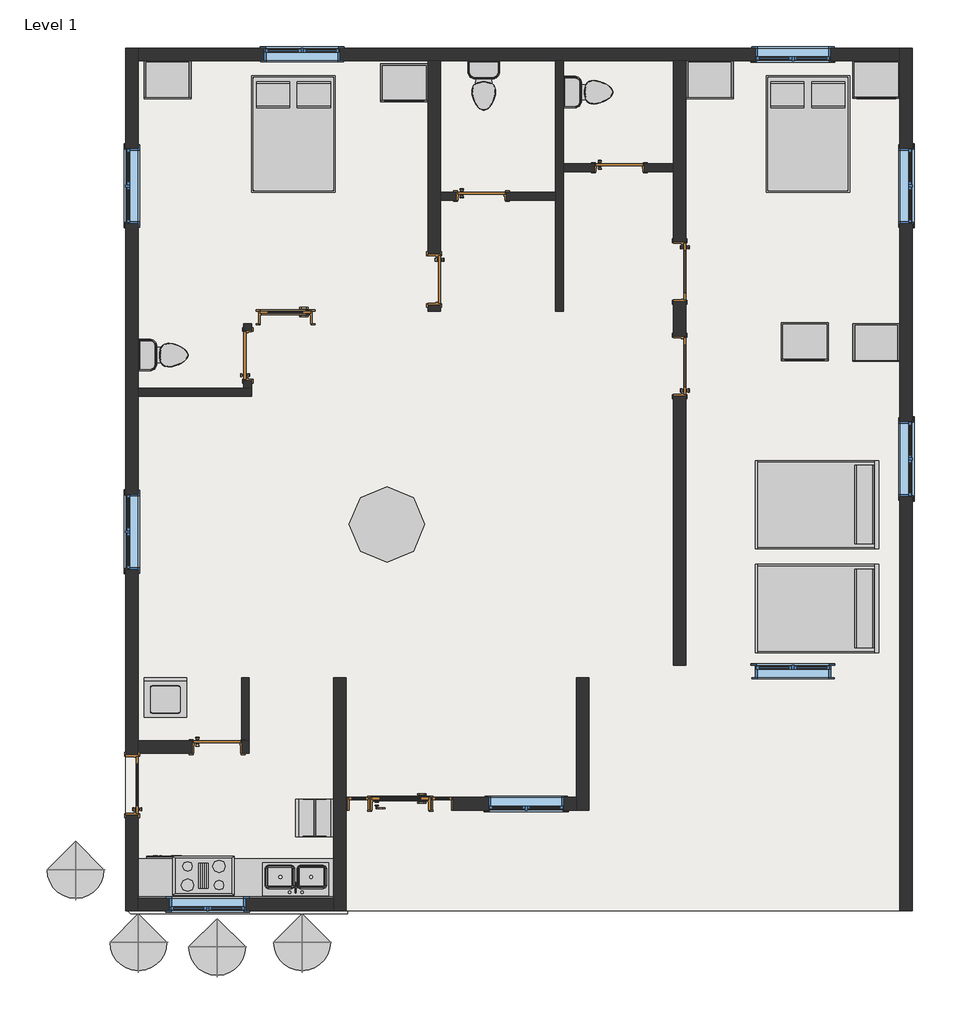
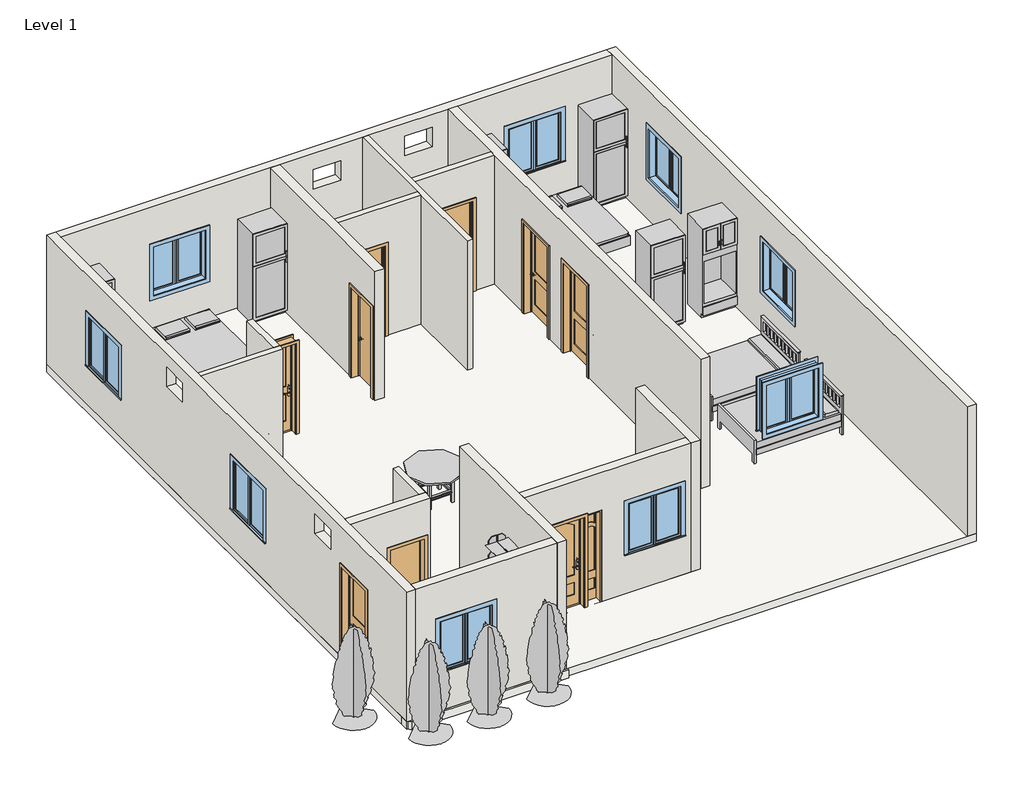
# One storey, incomplete: 16 walls, 13 doors, 12 furniture elements, 9 windows, 4 flow terminals, 4 geographic elements, 4 proxies, 3 slabs.
"""IFC4 building model written with IfcOpenShell, lengths in millimetres."""

from ifc_helpers import new_model, si_unit, frame, origin, place, context, project, spatial, polyline, outline, extrude, faceted_brep, transform, mapped, element, save
from components import proxy_a120491f, proxy_45b28599, proxy_279d5ef4, proxy_718fa39f, door_c3736dc5, door_823c627a, door_4a215221, door_6f959a6d, door_387d6dd4, door_interior_single_flush_panel_wood_df77f4d3, door_715cd483, entry_door_handle_standard_87575fd4, flow_terminal_a53be723, toilet_domestic_3d_toilet_domestic_3d_f7549cf7, toilet_domestic_3d_toilet_domestic_3d_183bbd19, furniture_c8abb964, furniture_096e7f55, furniture_23ec23c8, furniture_7060ebe6, furniture_fb6977ac, furniture_7f1a6afb, rpc_tree_conifer_chinese_juniper_7_1b9786cd, window_0862ab64, window_3a1167bf

model = new_model("IFC4")

# Units and contexts
model_context = context("Model", 3, world=origin())
ifc_project = project(units=[si_unit("LENGTHUNIT", "METRE", prefix="MILLI")], contexts=[model_context])

# Site, building, storey
site = spatial("IfcSite", under=ifc_project)
building = spatial("IfcBuilding", under=site)
storey = spatial("IfcBuildingStorey", under=building, Name="Level 1", Elevation=0.0)

# Proxies
placement = place(None, origin())
proxy_shape = proxy_a120491f(model_context)
element("IfcBuildingElementProxy", 1, Name="Cook Top-4 Unit : 42\" x 22\"", ObjectType="Cook Top-4 Unit : 42\" x 22\"", at=placement, inside=storey, context=model_context, shape_type="MappedRepresentation", body=[
    mapped(proxy_shape, transform((-17247.6111572, -428.8767698, 152.4), x_axis=(1.0, 0.0, 0.0), y_axis=(0.0, 1.0, 0.0), z_axis=(0.0, 0.0, 1.0))),
])
proxy_2_shape = proxy_45b28599(model_context)
element("IfcBuildingElementProxy", 2, Name="Dishwasher : 24\" x 24\" x 34\"", ObjectType="Dishwasher : 24\" x 24\" x 34\"", at=placement, inside=storey, context=model_context, shape_type="MappedRepresentation", body=[
    mapped(proxy_2_shape, transform((-17477.5286257, -168.2763346, 0.0), x_axis=(-1.0000000000000004, 0.0, 0.0), y_axis=(0.0, -1.0000000000000004, 0.0), z_axis=(0.0, 0.0, 1.0))),
])
proxy_3_shape = proxy_279d5ef4(model_context)
element("IfcBuildingElementProxy", 3, Name="Stack Shelving : 36\" x 90\"", ObjectType="Stack Shelving : 36\" x 90\"", at=placement, inside=storey, context=model_context, shape_type="MappedRepresentation", body=[
    mapped(proxy_3_shape, transform((-15450.5611572, 504.5732302, 0.0), x_axis=(0.0, 1.0000000000000002, 0.0), y_axis=(-1.0000000000000002, 0.0, 0.0), z_axis=(0.0, 0.0, 1.0))),
])
proxy_4_shape = proxy_718fa39f(model_context)
element("IfcBuildingElementProxy", 4, Name="Washer : 27\" x 25\" x 35\"", ObjectType="Washer : 27\" x 25\" x 35\"", at=placement, inside=storey, context=model_context, shape_type="MappedRepresentation", body=[
    mapped(proxy_4_shape, transform((-18280.2635627, 2168.5236654, 0.0), x_axis=(1.0, 0.0, 0.0), y_axis=(0.0, 1.0, 0.0), z_axis=(0.0, 0.0, 1.0))),
])

# Doors
door_shape = door_c3736dc5(model_context)
element("IfcDoor", 5, ObjectType="12\" x 84\"", at=placement, inside=storey, context=model_context, shape_type="MappedRepresentation", body=[
    mapped(door_shape, transform((-14739.3611572, 736.3482302, 0.0), x_axis=(1.0, 0.0, 0.0), y_axis=(0.0, 1.0, 0.0), z_axis=(0.0, 0.0, 1.0))),
])
element("IfcDoor", 6, ObjectType="12\" x 84\"", at=placement, inside=storey, context=model_context, shape_type="MappedRepresentation", body=[
    mapped(door_shape, transform((-13393.1611572, 736.3482302, 0.0), x_axis=(1.0, 0.0, 0.0), y_axis=(0.0, 1.0, 0.0), z_axis=(0.0, 0.0, 1.0))),
])
door_2_shape = door_823c627a(model_context)
element("IfcDoor", 7, ObjectType="32\" x 84\"", at=placement, inside=storey, context=model_context, shape_type="MappedRepresentation", body=[
    mapped(door_2_shape, transform((-15920.4611572, 8584.9482302, 0.0), x_axis=(1.0, 0.0, 0.0), y_axis=(0.0, 1.0, 0.0), z_axis=(0.0, 0.0, 1.0))),
])
door_3_shape = door_4a215221(model_context)
element("IfcDoor", 8, ObjectType="36\" x 84\"", at=placement, inside=storey, context=model_context, shape_type="MappedRepresentation", body=[
    mapped(door_3_shape, transform((-14066.2611572, 736.3482302, 0.0), x_axis=(1.0, 0.0, 0.0), y_axis=(0.0, 1.0, 0.0), z_axis=(0.0, 0.0, 1.0))),
])
door_4_shape = door_6f959a6d(model_context)
element("IfcDoor", 9, ObjectType="Door-Interior-Single-2_Panel-Wood : 36\" x 84\"", at=placement, inside=storey, context=model_context, shape_type="MappedRepresentation", body=[
    mapped(door_4_shape, transform((-9554.5861572, 9318.3732302, 0.0), x_axis=(0.0, -1.0, 0.0), y_axis=(1.0, 0.0, 0.0), z_axis=(0.0, 0.0, 1.0))),
])
door_5_shape = door_387d6dd4(model_context)
element("IfcDoor", 10, ObjectType="Door-Interior-Single-2_Panel-Wood : 36\" x 84\"", at=placement, inside=storey, context=model_context, shape_type="MappedRepresentation", body=[
    mapped(door_5_shape, transform((-9554.5861572, 7794.3732302, 0.0), x_axis=(0.0, 1.0, 0.0), y_axis=(-1.0, 0.0, 0.0), z_axis=(0.0, 0.0, 1.0))),
])
element("IfcDoor", 11, ObjectType="Door-Interior-Single-2_Panel-Wood : 36\" x 84\"", at=placement, inside=storey, context=model_context, shape_type="MappedRepresentation", body=[
    mapped(door_5_shape, transform((-18393.7861572, 1037.9732302, 0.0), x_axis=(0.0, 1.0, 0.0), y_axis=(-1.0, 0.0, 0.0), z_axis=(0.0, 0.0, 1.0))),
])
door_interior_single_flush_panel_wood_shape = door_interior_single_flush_panel_wood_df77f4d3(model_context)
element("IfcDoor", 12, ObjectType="Door-Interior-Single-Flush_Panel-Wood", at=placement, inside=storey, context=model_context, shape_type="MappedRepresentation", body=[
    mapped(door_interior_single_flush_panel_wood_shape, transform((-16533.2361572, 7965.8232302, 0.0), x_axis=(0.0, 1.0, 0.0), y_axis=(-1.0, 0.0, 0.0), z_axis=(0.0, 0.0, 1.0))),
])
element("IfcDoor", 13, ObjectType="Door-Interior-Single-Flush_Panel-Wood", at=placement, inside=storey, context=model_context, shape_type="MappedRepresentation", body=[
    mapped(door_interior_single_flush_panel_wood_shape, transform((-12758.1611572, 10540.7482302, 0.0), x_axis=(1.0, 0.0, 0.0), y_axis=(0.0, 1.0, 0.0), z_axis=(0.0, 0.0, 1.0))),
])
element("IfcDoor", 14, ObjectType="Door-Interior-Single-Flush_Panel-Wood", at=placement, inside=storey, context=model_context, shape_type="MappedRepresentation", body=[
    mapped(door_interior_single_flush_panel_wood_shape, transform((-10529.3111572, 10997.9482302, 0.0), x_axis=(1.0, 0.0, 0.0), y_axis=(0.0, 1.0, 0.0), z_axis=(0.0, 0.0, 1.0))),
])
door_6_shape = door_715cd483(model_context)
element("IfcDoor", 15, ObjectType="Door-Interior-Single-Flush_Panel-Wood", at=placement, inside=storey, context=model_context, shape_type="MappedRepresentation", body=[
    mapped(door_6_shape, transform((-13516.9861572, 9191.3732302, 0.0), x_axis=(0.0, -1.0, 0.0), y_axis=(1.0, 0.0, 0.0), z_axis=(0.0, 0.0, 1.0))),
])
element("IfcDoor", 16, ObjectType="Door-Interior-Single-Flush_Panel-Wood : 30\" x 84\"", at=placement, inside=storey, context=model_context, shape_type="MappedRepresentation", body=[
    mapped(door_6_shape, transform((-17025.3611572, 1650.7482302, 0.0), x_axis=(1.0, 0.0, 0.0), y_axis=(0.0, 1.0, 0.0), z_axis=(0.0, 0.0, 1.0))),
])
entry_door_handle_standard_shape = entry_door_handle_standard_87575fd4(model_context)
element("IfcDoor", 17, ObjectType="Entry Door Handle : Standard", at=placement, inside=storey, context=model_context, shape_type="MappedRepresentation", body=[
    mapped(entry_door_handle_standard_shape, transform((-14447.2611572, 733.1732302, 914.4), x_axis=(1.0, 0.0, 0.0), y_axis=(0.0, 1.0, 0.0), z_axis=(0.0, 0.0, 1.0))),
])

# Flow terminals
flow_terminal_shape = flow_terminal_a53be723(model_context)
element("IfcFlowTerminal", 18, ObjectType="Sink Kitchen-Double : 42\" x 21\"", at=placement, inside=storey, context=model_context, shape_type="MappedRepresentation", body=[
    mapped(flow_terminal_shape, transform((-15739.6719166, -483.6813687, 0.0), x_axis=(-1.0, 0.0, 0.0), y_axis=(0.0, -1.0, 0.0), z_axis=(0.0, 0.0, 1.0))),
])
toilet_domestic_3d_toilet_domestic_3d_shape = toilet_domestic_3d_toilet_domestic_3d_f7549cf7(model_context)
toilet_domestic_3d_toilet_domestic_3d_2_shape = toilet_domestic_3d_toilet_domestic_3d_183bbd19(model_context)
element("IfcFlowTerminal", 19, ObjectType="Toilet-Domestic-3D : Toilet-Domestic-3D", at=placement, inside=storey, context=model_context, shape_type="MappedRepresentation", body=[
    mapped(toilet_domestic_3d_toilet_domestic_3d_shape, transform((-17800.6651298, 7972.1732302, 0.0), x_axis=(0.0, 1.0000000000000002, 0.0), y_axis=(-1.0000000000000002, 0.0, 0.0), z_axis=(0.0, 0.0, 1.0))),
    mapped(toilet_domestic_3d_toilet_domestic_3d_2_shape, transform((-17800.6651298, 7972.1732302, 0.0), x_axis=(0.0, 1.0000000000000002, 0.0), y_axis=(-1.0000000000000002, 0.0, 0.0), z_axis=(0.0, 0.0, 1.0))),
])
element("IfcFlowTerminal", 20, ObjectType="Toilet-Domestic-3D : Toilet-Domestic-3D", at=placement, inside=storey, context=model_context, shape_type="MappedRepresentation", body=[
    mapped(toilet_domestic_3d_toilet_domestic_3d_shape, transform((-12720.0611572, 12227.2772028, 0.0), x_axis=(1.0000000000000007, 0.0, 0.0), y_axis=(0.0, 1.0000000000000007, 0.0), z_axis=(0.0, 0.0, 1.0))),
    mapped(toilet_domestic_3d_toilet_domestic_3d_2_shape, transform((-12720.0611572, 12227.2772028, 0.0), x_axis=(1.0000000000000007, 0.0, 0.0), y_axis=(0.0, 1.0000000000000007, 0.0), z_axis=(0.0, 0.0, 1.0))),
])
element("IfcFlowTerminal", 21, ObjectType="Toilet-Domestic-3D : Toilet-Domestic-3D", at=placement, inside=storey, context=model_context, shape_type="MappedRepresentation", body=[
    mapped(toilet_domestic_3d_toilet_domestic_3d_shape, transform((-10942.6651298, 12213.9732302, 0.0), x_axis=(0.0, 1.0000000000000002, 0.0), y_axis=(-1.0000000000000002, 0.0, 0.0), z_axis=(0.0, 0.0, 1.0))),
    mapped(toilet_domestic_3d_toilet_domestic_3d_2_shape, transform((-10942.6651298, 12213.9732302, 0.0), x_axis=(0.0, 1.0000000000000002, 0.0), y_axis=(-1.0000000000000002, 0.0, 0.0), z_axis=(0.0, 0.0, 1.0))),
])

# Furniture
furniture_shape = furniture_c8abb964(model_context)
element("IfcFurniture", 22, ObjectType="Bed-Box : Double 53\" x 74\"", at=placement, inside=storey, context=model_context, shape_type="MappedRepresentation", body=[
    mapped(furniture_shape, transform((-16132.6136162, 11775.3027384, 0.0), x_axis=(1.0, 0.0, 0.0), y_axis=(0.0, 1.0, 0.0), z_axis=(0.0, 0.0, 1.0))),
])
element("IfcFurniture", 23, ObjectType="Bed-Box : Double 53\" x 74\"", at=placement, inside=storey, context=model_context, shape_type="MappedRepresentation", body=[
    mapped(furniture_shape, transform((-7826.8136162, 11775.3027384, 0.0), x_axis=(1.0, 0.0, 0.0), y_axis=(0.0, 1.0, 0.0), z_axis=(0.0, 0.0, 1.0))),
])
furniture_2_shape = furniture_096e7f55(model_context)
element("IfcFurniture", 24, ObjectType="Bed-Shaker : Double 56\" x 78\"", at=placement, inside=storey, context=model_context, shape_type="MappedRepresentation", body=[
    mapped(furniture_2_shape, transform((-6357.3611572, 3863.7232302, 0.0), x_axis=(0.0, -1.0000000000000002, 0.0), y_axis=(1.0000000000000002, 0.0, 0.0), z_axis=(0.0, 0.0, 1.0))),
])
element("IfcFurniture", 25, ObjectType="Bed-Shaker : Double 56\" x 78\"", at=placement, inside=storey, context=model_context, shape_type="MappedRepresentation", body=[
    mapped(furniture_2_shape, transform((-6357.3611572, 5540.1232302, 0.0), x_axis=(0.0, -1.0000000000000002, 0.0), y_axis=(1.0000000000000002, 0.0, 0.0), z_axis=(0.0, 0.0, 1.0))),
])
furniture_3_shape = furniture_23ec23c8(model_context)
element("IfcFurniture", 26, ObjectType="Counter Top w Sink : 24\" Depth", at=placement, inside=storey, context=model_context, shape_type="MappedRepresentation", body=[
    mapped(furniture_3_shape, transform((-16346.2234522, -790.8267698, 0.0), x_axis=(-1.0, 0.0, 0.0), y_axis=(0.0, -1.0, 0.0), z_axis=(0.0, 0.0, 1.0))),
])
furniture_4_shape = furniture_7060ebe6(model_context)
element("IfcFurniture", 27, ObjectType="Table-Dining Round w Chairs : 36\" Diameter", at=placement, inside=storey, context=model_context, shape_type="MappedRepresentation", body=[
    mapped(furniture_4_shape, transform((-14385.8431244, 5426.5519187, 0.0), x_axis=(1.0, 0.0, 0.0), y_axis=(0.0, 1.0, 0.0), z_axis=(0.0, 0.0, 1.0))),
])
furniture_5_shape = furniture_fb6977ac(model_context)
element("IfcFurniture", 28, ObjectType="Tall Cabinet-2 Door-Built in : 30\"", at=placement, inside=storey, context=model_context, shape_type="MappedRepresentation", body=[
    mapped(furniture_5_shape, transform((-17844.1988621, 12721.9732302, 0.0), x_axis=(1.0, 0.0, 0.0), y_axis=(0.0, 1.0, 0.0), z_axis=(0.0, 0.0, 1.0))),
])
element("IfcFurniture", 29, ObjectType="Tall Cabinet-2 Door-Built in : 30\"", at=placement, inside=storey, context=model_context, shape_type="MappedRepresentation", body=[
    mapped(furniture_5_shape, transform((-9093.8988621, 12721.9732302, 0.0), x_axis=(1.0, 0.0, 0.0), y_axis=(0.0, 1.0, 0.0), z_axis=(0.0, 0.0, 1.0))),
])
element("IfcFurniture", 30, ObjectType="Tall Cabinet-2 Door-Built in : 30\"", at=placement, inside=storey, context=model_context, shape_type="MappedRepresentation", body=[
    mapped(furniture_5_shape, transform((-6401.4988621, 8480.1732302, 0.0), x_axis=(1.0, 0.0, 0.0), y_axis=(0.0, 1.0, 0.0), z_axis=(0.0, 0.0, 1.0))),
])
furniture_6_shape = furniture_7f1a6afb(model_context)
element("IfcFurniture", 31, ObjectType="Tall Cabinet-Single Door(2) : 30\"", at=placement, inside=storey, context=model_context, shape_type="MappedRepresentation", body=[
    mapped(furniture_6_shape, transform((-7557.1988621, 8492.8732302, 0.0), x_axis=(1.0000000000000002, 0.0, 0.0), y_axis=(0.0, 1.0000000000000002, 0.0), z_axis=(0.0, 0.0, 1.0))),
])
element("IfcFurniture", 32, ObjectType="Tall Cabinet-Single Door(2) : 30\"", at=placement, inside=storey, context=model_context, shape_type="MappedRepresentation", body=[
    mapped(furniture_6_shape, transform((-6401.4988621, 12721.9732302, 0.0), x_axis=(1.0, 0.0, 0.0), y_axis=(0.0, 1.0, 0.0), z_axis=(0.0, 0.0, 1.0))),
])
element("IfcFurniture", 33, ObjectType="Tall Cabinet-Single Door(2) : 30\"", at=placement, inside=storey, context=model_context, shape_type="MappedRepresentation", body=[
    mapped(furniture_6_shape, transform((-14021.4988621, 12671.1732302, 0.0), x_axis=(1.0, 0.0, 0.0), y_axis=(0.0, 1.0, 0.0), z_axis=(0.0, 0.0, 1.0))),
])

# Geographic elements
rpc_tree_conifer_chinese_juniper_7_shape = rpc_tree_conifer_chinese_juniper_7_1b9786cd(model_context)
element("IfcGeographicElement", 34, ObjectType="RPC Tree - Conifer : Chinese Juniper - 7'", at=placement, inside=storey, context=model_context, shape_type="MappedRepresentation", body=[
    mapped(rpc_tree_conifer_chinese_juniper_7_shape, transform((-18295.5578282, -1502.0267698, 0.0), x_axis=(1.0, 0.0, 0.0), y_axis=(0.0, 1.0, 0.0), z_axis=(0.0, 0.0, 1.0))),
])
element("IfcGeographicElement", 35, ObjectType="RPC Tree - Conifer : Chinese Juniper - 7'", at=placement, inside=storey, context=model_context, shape_type="MappedRepresentation", body=[
    mapped(rpc_tree_conifer_chinese_juniper_7_shape, transform((-17025.5578282, -1578.2267698, 0.0), x_axis=(1.0, 0.0, 0.0), y_axis=(0.0, 1.0, 0.0), z_axis=(0.0, 0.0, 1.0))),
])
element("IfcGeographicElement", 36, ObjectType="RPC Tree - Conifer : Chinese Juniper - 7'", at=placement, inside=storey, context=model_context, shape_type="MappedRepresentation", body=[
    mapped(rpc_tree_conifer_chinese_juniper_7_shape, transform((-15653.9578282, -1502.0267698, 0.0), x_axis=(1.0, 0.0, 0.0), y_axis=(0.0, 1.0, 0.0), z_axis=(0.0, 0.0, 1.0))),
])
element("IfcGeographicElement", 37, ObjectType="RPC Tree - Conifer : Chinese Juniper - 7'", at=placement, inside=storey, context=model_context, shape_type="MappedRepresentation", body=[
    mapped(rpc_tree_conifer_chinese_juniper_7_shape, transform((-19311.5578282, -333.6267698, 0.0), x_axis=(1.0, 0.0, 0.0), y_axis=(0.0, 1.0, 0.0), z_axis=(0.0, 0.0, 1.0))),
])

# Slabs
element("IfcSlab", 38, ObjectType="Generic - 12\"", at=placement, inside=storey, context=model_context, shape_type="SweptSolid", body=[
    extrude(outline(polyline([(-5798.5611572, 12925.1732302), (-5798.5611572, -790.8267698), (-5798.5611572, -994.0267698), (-18498.5611572, -994.0267698), (-18498.5611572, -790.8267698), (-18498.5611572, 12925.1732302), (-5798.5611572, 12925.1732302)])), frame((0.0, 0.0, -182.8601563), z_axis=(0.0, 0.0, 1.0), x_axis=(1.0, 0.0, 0.0)), (0.0, 0.0, 1.0), 182.8601563),
])
element("IfcSlab", 39, ObjectType="Generic - 12\"", at=placement, inside=storey, context=model_context, shape_type="SweptSolid", body=[
    extrude(outline(polyline([(-5798.5611572, 12925.1732302), (-5798.5611572, 2765.1732302), (-11018.2611572, 2765.1732302), (-11018.2611572, 631.5732302), (-14917.1611572, 631.5732302), (-14917.1611572, -1044.8267698), (-18422.3611572, -1044.8267698), (-18498.5611572, -968.6267698), (-18498.5611572, 12925.1732302), (-5798.5611572, 12925.1732302)])), frame((0.0, 0.0, -182.8601563), z_axis=(0.0, 0.0, 1.0), x_axis=(1.0, 0.0, 0.0)), (0.0, 0.0, 1.0), 182.8601563),
])
element("IfcSlab", 40, ObjectType="Generic - 12\"", at=placement, inside=storey, context=model_context, shape_type="SweptSolid", body=[
    extrude(outline(polyline([(-5798.5611572, 12925.1732302), (-5798.5611572, 2765.1732302), (-18498.5611572, 2765.1732302), (-18498.5611572, 12925.1732302), (-5798.5611572, 12925.1732302)])), frame((0.0, 0.0, -182.8601563), z_axis=(0.0, 0.0, 1.0), x_axis=(1.0, 0.0, 0.0)), (0.0, 0.0, 1.0), 182.8601563),
])

# Walls
element("IfcWall", 41, at=placement, inside=storey, context=model_context, shape_type="Brep", body=[
    faceted_brep([(-18295.3611572, 12721.9732302, 0.0), (-13621.7611572, 12721.9732302, 0.0), (-13418.5611572, 12721.9732302, 0.0), (-11564.3611572, 12721.9732302, 0.0), (-11437.3611572, 12721.9732302, 0.0), (-9659.3611572, 12721.9732302, 0.0), (-9456.1611572, 12721.9732302, 0.0), (-6001.7611572, 12721.9732302, 0.0), (-6001.7611572, 12721.9732302, 3048.0), (-9456.1611572, 12721.9732302, 3048.0), (-9659.3611572, 12721.9732302, 3048.0), (-11437.3611572, 12721.9732302, 3048.0), (-11564.3611572, 12721.9732302, 3048.0), (-13418.5611572, 12721.9732302, 3048.0), (-13621.7611572, 12721.9732302, 3048.0), (-18295.3611572, 12721.9732302, 3048.0), (-16263.3611572, 12721.9732302, 2133.6), (-15044.1611572, 12721.9732302, 2133.6), (-15044.1611572, 12721.9732302, 914.4), (-16263.3611572, 12721.9732302, 914.4), (-8338.5611572, 12721.9732302, 2133.6), (-7119.3611572, 12721.9732302, 2133.6), (-7119.3611572, 12721.9732302, 914.4), (-8338.5611572, 12721.9732302, 914.4), (-12053.3111572, 12721.9732302, 2667.0), (-12053.3111572, 12721.9732302, 2209.8), (-12662.9111572, 12721.9732302, 2209.8), (-12662.9111572, 12721.9732302, 2667.0), (-10624.5611572, 12721.9732302, 2743.2), (-10014.9611572, 12721.9732302, 2743.2), (-10014.9611572, 12721.9732302, 2286.0), (-10624.5611572, 12721.9732302, 2286.0), (-18295.3611572, 12925.1732302, 0.0), (-18295.3611572, 12925.1732302, 3048.0), (-6001.7611572, 12925.1732302, 3048.0), (-6001.7611572, 12925.1732302, 0.0), (-16263.3611572, 12925.1732302, 2133.6), (-16263.3611572, 12925.1732302, 914.4), (-15044.1611572, 12925.1732302, 914.4), (-15044.1611572, 12925.1732302, 2133.6), (-8338.5611572, 12925.1732302, 2133.6), (-8338.5611572, 12925.1732302, 914.4), (-7119.3611572, 12925.1732302, 914.4), (-7119.3611572, 12925.1732302, 2133.6), (-12053.3111572, 12925.1732302, 2667.0), (-12662.9111572, 12925.1732302, 2667.0), (-12662.9111572, 12925.1732302, 2209.8), (-12053.3111572, 12925.1732302, 2209.8), (-10624.5611572, 12925.1732302, 2743.2), (-10624.5611572, 12925.1732302, 2286.0), (-10014.9611572, 12925.1732302, 2286.0), (-10014.9611572, 12925.1732302, 2743.2)], [[[0, 1, 2, 3, 4, 5, 6, 7, 8, 9, 10, 11, 12, 13, 14, 15], [16, 17, 18, 19], [20, 21, 22, 23], [24, 25, 26, 27], [28, 29, 30, 31]], [[32, 33, 34, 35], [36, 37, 38, 39], [40, 41, 42, 43], [44, 45, 46, 47], [48, 49, 50, 51]], [[7, 6, 5, 4, 3, 2, 1, 0, 32, 35]], [[15, 14, 13, 12, 11, 10, 9, 8, 34, 33]], [[0, 15, 33, 32]], [[8, 7, 35, 34]], [[37, 36, 16, 19]], [[38, 37, 19, 18]], [[39, 38, 18, 17]], [[36, 39, 17, 16]], [[41, 40, 20, 23]], [[42, 41, 23, 22]], [[43, 42, 22, 21]], [[40, 43, 21, 20]], [[25, 24, 44, 47]], [[26, 25, 47, 46]], [[27, 26, 46, 45]], [[24, 27, 45, 44]], [[49, 48, 28, 31]], [[50, 49, 31, 30]], [[51, 50, 30, 29]], [[48, 51, 29, 28]]]),
])
element("IfcWall", 42, at=placement, inside=storey, context=model_context, shape_type="Brep", body=[
    faceted_brep([(-6001.7611572, 12925.1732302, 0.0), (-6001.7611572, 12721.9732302, 0.0), (-6001.7611572, 8683.3732302, 0.0), (-6001.7611572, 8480.1732302, 0.0), (-6001.7611572, 2968.3732302, 0.0), (-6001.7611572, 2765.1732302, 0.0), (-6001.7611572, -994.0267698, 0.0), (-6001.7611572, -994.0267698, 3048.0), (-6001.7611572, 2765.1732302, 3048.0), (-6001.7611572, 2968.3732302, 3048.0), (-6001.7611572, 8480.1732302, 3048.0), (-6001.7611572, 8683.3732302, 3048.0), (-6001.7611572, 12721.9732302, 3048.0), (-6001.7611572, 12925.1732302, 3048.0), (-6001.7611572, 10093.0732302, 2209.8), (-6001.7611572, 10093.0732302, 990.6), (-6001.7611572, 11312.2732302, 990.6), (-6001.7611572, 11312.2732302, 2209.8), (-6001.7611572, 5686.1732302, 2209.8), (-6001.7611572, 5686.1732302, 990.6), (-6001.7611572, 6905.3732302, 990.6), (-6001.7611572, 6905.3732302, 2209.8), (-5798.5611572, 12925.1732302, 0.0), (-5798.5611572, 12925.1732302, 3048.0), (-5798.5611572, -994.0267698, 3048.0), (-5798.5611572, -994.0267698, 0.0), (-5798.5611572, 10093.0732302, 2209.8), (-5798.5611572, 11312.2732302, 2209.8), (-5798.5611572, 11312.2732302, 990.6), (-5798.5611572, 10093.0732302, 990.6), (-5798.5611572, 5686.1732302, 2209.8), (-5798.5611572, 6905.3732302, 2209.8), (-5798.5611572, 6905.3732302, 990.6), (-5798.5611572, 5686.1732302, 990.6)], [[[0, 1, 2, 3, 4, 5, 6, 7, 8, 9, 10, 11, 12, 13], [14, 15, 16, 17], [18, 19, 20, 21]], [[22, 23, 24, 25], [26, 27, 28, 29], [30, 31, 32, 33]], [[6, 5, 4, 3, 2, 1, 0, 22, 25]], [[7, 6, 25, 24]], [[13, 12, 11, 10, 9, 8, 7, 24, 23]], [[0, 13, 23, 22]], [[15, 14, 26, 29]], [[16, 15, 29, 28]], [[17, 16, 28, 27]], [[14, 17, 27, 26]], [[19, 18, 30, 33]], [[20, 19, 33, 32]], [[21, 20, 32, 31]], [[18, 21, 31, 30]]]),
])
element("IfcWall", 43, ObjectType="Generic - 5\"", at=placement, inside=storey, context=model_context, shape_type="Brep", body=[
    faceted_brep([(-11564.3611572, 12721.9732302, 0.0), (-11564.3611572, 10601.0732302, 0.0), (-11564.3611572, 10474.0732302, 0.0), (-11564.3611572, 8683.3732302, 0.0), (-11564.3611572, 8683.3732302, 3048.0), (-11564.3611572, 10474.0732302, 3048.0), (-11564.3611572, 10601.0732302, 3048.0), (-11564.3611572, 12721.9732302, 3048.0), (-11437.3611572, 12721.9732302, 0.0), (-11437.3611572, 12721.9732302, 3048.0), (-11437.3611572, 11058.2732302, 3048.0), (-11437.3611572, 10931.2732302, 3048.0), (-11437.3611572, 8683.3732302, 3048.0), (-11437.3611572, 8683.3732302, 1325.7615426), (-11437.3611572, 8683.3732302, 0.0), (-11437.3611572, 10931.2732302, 0.0), (-11437.3611572, 11058.2732302, 0.0)], [[[0, 1, 2, 3, 4, 5, 6, 7]], [[8, 9, 10, 11, 12, 13, 14, 15, 16]], [[3, 2, 1, 0, 8, 16, 15, 14]], [[7, 6, 5, 4, 12, 11, 10, 9]], [[0, 7, 9, 8]], [[3, 14, 13, 12, 4]]]),
])
element("IfcWall", 44, ObjectType="Generic - 5\"", at=placement, inside=storey, context=model_context, shape_type="Brep", body=[
    faceted_brep([(-18295.3611572, 7311.7732302, 0.0), (-16466.5611572, 7311.7732302, 0.0), (-16466.5611572, 7311.7732302, 3048.0), (-18295.3611572, 7311.7732302, 3048.0), (-18295.3611572, 7438.7732302, 0.0), (-18295.3611572, 7438.7732302, 3048.0), (-16593.5611572, 7438.7732302, 3048.0), (-16466.5611572, 7438.7732302, 3048.0), (-16466.5611572, 7438.7732302, 0.0), (-16593.5611572, 7438.7732302, 0.0)], [[[0, 1, 2, 3]], [[4, 5, 6, 7, 8, 9]], [[1, 0, 4, 9, 8]], [[3, 2, 7, 6, 5]], [[0, 3, 5, 4]], [[2, 1, 8, 7]]]),
])
element("IfcWall", 45, ObjectType="Generic - 5\"", at=placement, inside=storey, context=model_context, shape_type="SweptSolid", body=[
    extrude(outline(polyline([(7438.7732302, 3048.0), (8480.1732302, 3048.0), (8480.1732302, 0.0), (8372.2232302, 0.0), (8372.2232302, 2159.0), (7559.4232302, 2159.0), (7559.4232302, 0.0), (7438.7732302, 0.0), (7438.7732302, 3048.0)])), frame((-16593.5611572, 0.0, 0.0), z_axis=(1.0, 0.0, 0.0), x_axis=(0.0, 1.0, 0.0)), (0.0, 0.0, 1.0), 127.0),
])
element("IfcWall", 46, ObjectType="Generic - 5\"", at=placement, inside=storey, context=model_context, shape_type="Brep", body=[
    faceted_brep([(-16631.6611572, 2765.1732302, 0.0), (-16631.6611572, 1749.1732302, 0.0), (-16631.6611572, 1749.1732302, 3048.0), (-16631.6611572, 2765.1732302, 3048.0), (-16504.6611572, 2765.1732302, 0.0), (-16504.6611572, 2765.1732302, 3048.0), (-16504.6611572, 1749.1732302, 3048.0), (-16504.6611572, 1749.1732302, 0.0), (-16618.9611572, 1749.1732302, 0.0)], [[[0, 1, 2, 3]], [[4, 5, 6, 7]], [[1, 0, 4, 7, 8]], [[3, 2, 6, 5]], [[2, 1, 8, 7, 6]], [[0, 3, 5, 4]]]),
])
element("IfcWall", 47, ObjectType="Generic - 5\"", at=placement, inside=storey, context=model_context, shape_type="SweptSolid", body=[
    extrude(outline(polyline([(3048.0, -9659.3611572), (3048.0, -11437.3611572), (0.0, -11437.3611572), (0.0, -10935.7111572), (2159.0, -10935.7111572), (2159.0, -10122.9111572), (0.0, -10122.9111572), (0.0, -9659.3611572), (3048.0, -9659.3611572)])), frame((0.0, 10931.2732302, 0.0), z_axis=(0.0, 1.0, 0.0), x_axis=(0.0, 0.0, 1.0)), (0.0, 0.0, 1.0), 127.0),
])
element("IfcWall", 48, ObjectType="Generic - 5\"", at=placement, inside=storey, context=model_context, shape_type="SweptSolid", body=[
    extrude(outline(polyline([(3048.0, -11564.3611572), (3048.0, -13418.5611572), (0.0, -13418.5611572), (0.0, -13164.5611572), (2159.0, -13164.5611572), (2159.0, -12351.7611572), (0.0, -12351.7611572), (0.0, -11564.3611572), (3048.0, -11564.3611572)])), frame((0.0, 10474.0732302, 0.0), z_axis=(0.0, 1.0, 0.0), x_axis=(0.0, 0.0, 1.0)), (0.0, 0.0, 1.0), 127.0),
])
element("IfcWall", 49, ObjectType="Generic - 8\"", at=placement, inside=storey, context=model_context, shape_type="Brep", body=[
    faceted_brep([(-13621.7611572, 8683.3732302, 3048.0), (-13621.7611572, 12721.9732302, 3048.0), (-13621.7611572, 12721.9732302, 0.0), (-13621.7611572, 9597.7732302, 0.0), (-13621.7611572, 9597.7732302, 2159.0), (-13621.7611572, 8784.9732302, 2159.0), (-13621.7611572, 8784.9732302, 0.0), (-13621.7611572, 8683.3732302, 0.0), (-13418.5611572, 12721.9732302, 3048.0), (-13418.5611572, 10601.0732302, 3048.0), (-13418.5611572, 10474.0732302, 3048.0), (-13418.5611572, 8683.3732302, 3048.0), (-13418.5611572, 8683.3732302, 0.0), (-13418.5611572, 8784.9732302, 0.0), (-13418.5611572, 8784.9732302, 2159.0), (-13418.5611572, 9597.7732302, 2159.0), (-13418.5611572, 9597.7732302, 0.0), (-13418.5611572, 10474.0732302, 0.0), (-13418.5611572, 10601.0732302, 0.0), (-13418.5611572, 12721.9732302, 0.0)], [[[0, 1, 2, 3, 4, 5, 6, 7]], [[8, 9, 10, 11, 12, 13, 14, 15, 16, 17, 18, 19]], [[2, 19, 18, 17, 16, 3]], [[12, 7, 6, 13]], [[1, 0, 11, 10, 9, 8]], [[2, 1, 8, 19]], [[0, 7, 12, 11]], [[5, 14, 13, 6]], [[14, 5, 4, 15]], [[15, 4, 3, 16]]]),
])
element("IfcWall", 50, ObjectType="Generic - 8\"", at=placement, inside=storey, context=model_context, shape_type="Brep", body=[
    faceted_brep([(-9659.3611572, 2968.3732302, 3048.0), (-9659.3611572, 8280.1770962, 3048.0), (-9659.3611572, 8454.7732302, 3048.0), (-9659.3611572, 8480.1732302, 3048.0), (-9659.3611572, 10931.2732302, 3048.0), (-9659.3611572, 11058.2732302, 3048.0), (-9659.3611572, 12721.9732302, 3048.0), (-9659.3611572, 12721.9732302, 0.0), (-9659.3611572, 11058.2732302, 0.0), (-9659.3611572, 10931.2732302, 0.0), (-9659.3611572, 9800.9732302, 0.0), (-9659.3611572, 9800.9732302, 2159.0), (-9659.3611572, 8835.7732302, 2159.0), (-9659.3611572, 8835.7732302, 0.0), (-9659.3611572, 8556.3732302, 0.0), (-9659.3611572, 8454.7732302, 0.0), (-9659.3611572, 8353.1732302, 0.0), (-9659.3611572, 8276.9732302, 0.0), (-9659.3611572, 8276.9732302, 2159.0), (-9659.3611572, 7311.7732302, 2159.0), (-9659.3611572, 7311.7732302, 0.0), (-9659.3611572, 2968.3732302, 0.0), (-9456.1611572, 12721.9732302, 3048.0), (-9456.1611572, 2968.3732302, 3048.0), (-9456.1611572, 2968.3732302, 0.0), (-9456.1611572, 7311.7732302, 0.0), (-9456.1611572, 7311.7732302, 2159.0), (-9456.1611572, 8276.9732302, 2159.0), (-9456.1611572, 8276.9732302, 0.0), (-9456.1611572, 8835.7732302, 0.0), (-9456.1611572, 8835.7732302, 2159.0), (-9456.1611572, 9800.9732302, 2159.0), (-9456.1611572, 9800.9732302, 0.0), (-9456.1611572, 12721.9732302, 0.0)], [[[0, 1, 2, 3, 4, 5, 6, 7, 8, 9, 10, 11, 12, 13, 14, 15, 16, 17, 18, 19, 20, 21]], [[22, 23, 24, 25, 26, 27, 28, 29, 30, 31, 32, 33]], [[7, 6, 22, 33]], [[0, 21, 24, 23]], [[12, 30, 29, 13]], [[30, 12, 11, 31]], [[31, 11, 10, 32]], [[27, 18, 17, 28]], [[18, 27, 26, 19]], [[19, 26, 25, 20]], [[10, 9, 8, 7, 33, 32]], [[13, 29, 28, 17, 16, 15, 14]], [[24, 21, 20, 25]], [[6, 5, 4, 3, 2, 1, 0, 23, 22]]]),
])
element("IfcWall", 51, ObjectType="Generic - 8\"", at=placement, inside=storey, context=model_context, shape_type="Brep", body=[
    faceted_brep([(-15145.7611572, 2765.1732302, 0.0), (-15145.7611572, -790.8267698, 0.0), (-15145.7611572, -994.0267698, 0.0), (-15145.7611572, -994.0267698, 3048.0), (-15145.7611572, -790.8267698, 3048.0), (-15145.7611572, 2765.1732302, 3048.0), (-14942.5611572, 2765.1732302, 0.0), (-14942.5611572, 2765.1732302, 3048.0), (-14942.5611572, 834.7732302, 3048.0), (-14942.5611572, 631.5732302, 3048.0), (-14942.5611572, -994.0267698, 3048.0), (-14942.5611572, -994.0267698, 0.0), (-14942.5611572, 631.5732302, 0.0), (-14942.5611572, 834.7732302, 0.0)], [[[0, 1, 2, 3, 4, 5]], [[6, 7, 8, 9, 10, 11, 12, 13]], [[2, 1, 0, 6, 13, 12, 11]], [[5, 4, 3, 10, 9, 8, 7]], [[3, 2, 11, 10]], [[0, 5, 7, 6]]]),
])
element("IfcWall", 52, ObjectType="Generic - 8\"", at=placement, inside=storey, context=model_context, shape_type="Brep", body=[
    faceted_brep([(-16504.6611572, 1545.9732302, 3048.0), (-18295.3611572, 1545.9732302, 3048.0), (-18295.3611572, 1545.9732302, 0.0), (-17431.7611572, 1545.9732302, 0.0), (-17431.7611572, 1545.9732302, 2159.0), (-16618.9611572, 1545.9732302, 2159.0), (-16618.9611572, 1545.9732302, 0.0), (-16504.6611572, 1545.9732302, 0.0), (-18295.3611572, 1749.1732302, 3048.0), (-16631.6611572, 1749.1732302, 3048.0), (-16504.6611572, 1749.1732302, 3048.0), (-16504.6611572, 1749.1732302, 0.0), (-16618.9611572, 1749.1732302, 0.0), (-16618.9611572, 1749.1732302, 2159.0), (-17431.7611572, 1749.1732302, 2159.0), (-17431.7611572, 1749.1732302, 0.0), (-18295.3611572, 1749.1732302, 0.0)], [[[0, 1, 2, 3, 4, 5, 6, 7]], [[8, 9, 10, 11, 12, 13, 14, 15, 16]], [[2, 16, 15, 3]], [[11, 7, 6, 12]], [[1, 0, 10, 9, 8]], [[2, 1, 8, 16]], [[0, 7, 11, 10]], [[5, 13, 12, 6]], [[13, 5, 4, 14]], [[14, 4, 3, 15]]]),
])
element("IfcWall", 53, ObjectType="a", at=placement, inside=storey, context=model_context, shape_type="Brep", body=[
    faceted_brep([(-18498.5611572, -994.0267698, 3048.0), (-18498.5611572, 12925.1732302, 3048.0), (-18498.5611572, 12925.1732302, 0.0), (-18498.5611572, 1520.5732302, 0.0), (-18498.5611572, 1520.5732302, 2159.0), (-18498.5611572, 555.3732302, 2159.0), (-18498.5611572, 555.3732302, 0.0), (-18498.5611572, -994.0267698, 0.0), (-18498.5611572, 5730.6232302, 2133.6), (-18498.5611572, 4511.4232302, 2133.6), (-18498.5611572, 4511.4232302, 914.4), (-18498.5611572, 5730.6232302, 914.4), (-18498.5611572, 11312.2732302, 2133.6), (-18498.5611572, 10093.0732302, 2133.6), (-18498.5611572, 10093.0732302, 914.4), (-18498.5611572, 11312.2732302, 914.4), (-18498.5611572, 8283.3232302, 2743.2), (-18498.5611572, 7673.7232302, 2743.2), (-18498.5611572, 7673.7232302, 2286.0), (-18498.5611572, 8283.3232302, 2286.0), (-18498.5611572, 2561.9732302, 2743.2), (-18498.5611572, 1952.3732302, 2743.2), (-18498.5611572, 1952.3732302, 2286.0), (-18498.5611572, 2561.9732302, 2286.0), (-18295.3611572, 12925.1732302, 3048.0), (-18295.3611572, 12721.9732302, 3048.0), (-18295.3611572, 8683.3732302, 3048.0), (-18295.3611572, 8480.1732302, 3048.0), (-18295.3611572, 7438.7732302, 3048.0), (-18295.3611572, 7311.7732302, 3048.0), (-18295.3611572, 2968.3732302, 3048.0), (-18295.3611572, 2765.1732302, 3048.0), (-18295.3611572, 1749.1732302, 3048.0), (-18295.3611572, 1545.9732302, 3048.0), (-18295.3611572, -790.8267698, 3048.0), (-18295.3611572, -994.0267698, 3048.0), (-18295.3611572, -994.0267698, 0.0), (-18295.3611572, -790.8267698, 0.0), (-18295.3611572, 555.3732302, 0.0), (-18295.3611572, 555.3732302, 2159.0), (-18295.3611572, 1520.5732302, 2159.0), (-18295.3611572, 1520.5732302, 0.0), (-18295.3611572, 1545.9732302, 0.0), (-18295.3611572, 1749.1732302, 0.0), (-18295.3611572, 2765.1732302, 0.0), (-18295.3611572, 2968.3732302, 0.0), (-18295.3611572, 7311.7732302, 0.0), (-18295.3611572, 7438.7732302, 0.0), (-18295.3611572, 8480.1732302, 0.0), (-18295.3611572, 8683.3732302, 0.0), (-18295.3611572, 12721.9732302, 0.0), (-18295.3611572, 12925.1732302, 0.0), (-18295.3611572, 5730.6232302, 2133.6), (-18295.3611572, 5730.6232302, 914.4), (-18295.3611572, 4511.4232302, 914.4), (-18295.3611572, 4511.4232302, 2133.6), (-18295.3611572, 11312.2732302, 2133.6), (-18295.3611572, 11312.2732302, 914.4), (-18295.3611572, 10093.0732302, 914.4), (-18295.3611572, 10093.0732302, 2133.6), (-18295.3611572, 8283.3232302, 2743.2), (-18295.3611572, 8283.3232302, 2286.0), (-18295.3611572, 7673.7232302, 2286.0), (-18295.3611572, 7673.7232302, 2743.2), (-18295.3611572, 2561.9732302, 2743.2), (-18295.3611572, 2561.9732302, 2286.0), (-18295.3611572, 1952.3732302, 2286.0), (-18295.3611572, 1952.3732302, 2743.2)], [[[0, 1, 2, 3, 4, 5, 6, 7], [8, 9, 10, 11], [12, 13, 14, 15], [16, 17, 18, 19], [20, 21, 22, 23]], [[24, 25, 26, 27, 28, 29, 30, 31, 32, 33, 34, 35, 36, 37, 38, 39, 40, 41, 42, 43, 44, 45, 46, 47, 48, 49, 50, 51], [52, 53, 54, 55], [56, 57, 58, 59], [60, 61, 62, 63], [64, 65, 66, 67]], [[2, 51, 50, 49, 48, 47, 46, 45, 44, 43, 42, 41, 3]], [[36, 7, 6, 38, 37]], [[1, 0, 35, 34, 33, 32, 31, 30, 29, 28, 27, 26, 25, 24]], [[2, 1, 24, 51]], [[0, 7, 36, 35]], [[40, 4, 3, 41]], [[4, 40, 39, 5]], [[5, 39, 38, 6]], [[53, 52, 8, 11]], [[54, 53, 11, 10]], [[55, 54, 10, 9]], [[52, 55, 9, 8]], [[57, 56, 12, 15]], [[58, 57, 15, 14]], [[59, 58, 14, 13]], [[56, 59, 13, 12]], [[61, 60, 16, 19]], [[62, 61, 19, 18]], [[63, 62, 18, 17]], [[60, 63, 17, 16]], [[65, 64, 20, 23]], [[66, 65, 23, 22]], [[67, 66, 22, 21]], [[64, 67, 21, 20]]]),
])
element("IfcWall", 54, ObjectType="aw", at=placement, inside=storey, context=model_context, shape_type="SweptSolid", body=[
    extrude(outline(polyline([(0.0, -18295.3611572), (0.0, -15145.7611572), (3048.0, -15145.7611572), (3048.0, -18295.3611572), (0.0, -18295.3611572)]), holes=[polyline([(2133.6, -17787.3611572), (2133.6, -16568.1611572), (914.4, -16568.1611572), (914.4, -17787.3611572), (2133.6, -17787.3611572)])]), frame((0.0, -994.0267698, 0.0), z_axis=(0.0, 1.0, 0.0), x_axis=(0.0, 0.0, 1.0)), (0.0, 0.0, 1.0), 203.2),
])
element("IfcWall", 55, ObjectType="dq", at=placement, inside=storey, context=model_context, shape_type="Brep", body=[
    faceted_brep([(-11221.4611572, 2765.1732302, 0.0), (-11221.4611572, 834.7732302, 0.0), (-11221.4611572, 631.5732302, 0.0), (-11221.4611572, 631.5732302, 3048.0), (-11221.4611572, 834.7732302, 3048.0), (-11221.4611572, 2765.1732302, 3048.0), (-11018.2611572, 2765.1732302, 0.0), (-11018.2611572, 2765.1732302, 3048.0), (-11018.2611572, 631.5732302, 3048.0), (-11018.2611572, 631.5732302, 0.0)], [[[0, 1, 2, 3, 4, 5]], [[6, 7, 8, 9]], [[2, 1, 0, 6, 9]], [[5, 4, 3, 8, 7]], [[0, 5, 7, 6]], [[3, 2, 9, 8]]]),
])
element("IfcWall", 56, ObjectType="dq", at=placement, inside=storey, context=model_context, shape_type="SweptSolid", body=[
    extrude(outline(polyline([(3048.0, -11221.4611572), (3048.0, -14942.5611572), (0.0, -14942.5611572), (0.0, -14917.1611572), (2159.0, -14917.1611572), (2159.0, -14561.5611572), (0.0, -14561.5611572), (0.0, -14548.8611572), (2159.0, -14548.8611572), (2159.0, -13583.6611572), (0.0, -13583.6611572), (0.0, -13570.9611572), (2159.0, -13570.9611572), (2159.0, -13215.3611572), (0.0, -13215.3611572), (0.0, -11221.4611572), (3048.0, -11221.4611572)]), holes=[polyline([(2133.6, -12643.8611572), (2133.6, -11424.6611572), (914.4, -11424.6611572), (914.4, -12643.8611572), (2133.6, -12643.8611572)])]), frame((0.0, 631.5732302, 0.0), z_axis=(0.0, 1.0, 0.0), x_axis=(0.0, 0.0, 1.0)), (0.0, 0.0, 1.0), 203.2),
])

# Windows
window_shape = window_0862ab64(model_context)
element("IfcWindow", 57, ObjectType="Casement Dbl with Trim : 48\" x 48\"", at=placement, inside=storey, context=model_context, shape_type="MappedRepresentation", body=[
    mapped(window_shape, transform((-5919.2111572, 10702.6732302, 76.2), x_axis=(0.0, -1.0, 0.0), y_axis=(1.0, 0.0, 0.0), z_axis=(0.0, 0.0, 1.0))),
])
element("IfcWindow", 58, ObjectType="Casement Dbl with Trim : 48\" x 48\"", at=placement, inside=storey, context=model_context, shape_type="MappedRepresentation", body=[
    mapped(window_shape, transform((-5919.2111572, 6295.7732302, 76.2), x_axis=(0.0, -1.0, 0.0), y_axis=(1.0, 0.0, 0.0), z_axis=(0.0, 0.0, 1.0))),
])
element("IfcWindow", 59, ObjectType="Casement Dbl with Trim : 48\" x 48\"", at=placement, inside=storey, context=model_context, shape_type="MappedRepresentation", body=[
    mapped(window_shape, transform((-7728.9611572, 12842.6232302, 0.0), x_axis=(-1.0, 0.0, 0.0), y_axis=(0.0, -1.0, 0.0), z_axis=(0.0, 0.0, 1.0))),
])
window_2_shape = window_3a1167bf(model_context)
element("IfcWindow", 60, ObjectType="Casement Dbl with Trim : 48\" x 48\"", at=placement, inside=storey, context=model_context, shape_type="MappedRepresentation", body=[
    mapped(window_2_shape, transform((-15653.7611572, 12804.5232302, 0.0), x_axis=(-1.0, 0.0, 0.0), y_axis=(0.0, -1.0, 0.0), z_axis=(0.0, 0.0, 1.0))),
])
element("IfcWindow", 61, ObjectType="Casement Dbl with Trim : 48\" x 48\"", at=placement, inside=storey, context=model_context, shape_type="MappedRepresentation", body=[
    mapped(window_shape, transform((-18377.9111572, 5121.0232302, 0.0), x_axis=(0.0, 1.0, 0.0), y_axis=(-1.0, 0.0, 0.0), z_axis=(0.0, 0.0, 1.0))),
])
element("IfcWindow", 62, ObjectType="Casement Dbl with Trim : 48\" x 48\"", at=placement, inside=storey, context=model_context, shape_type="MappedRepresentation", body=[
    mapped(window_shape, transform((-18377.9111572, 10702.6732302, 0.0), x_axis=(0.0, 1.0, 0.0), y_axis=(-1.0, 0.0, 0.0), z_axis=(0.0, 0.0, 1.0))),
])
element("IfcWindow", 63, ObjectType="Casement Dbl with Trim : 48\" x 48\"", at=placement, inside=storey, context=model_context, shape_type="MappedRepresentation", body=[
    mapped(window_shape, transform((-17177.7611572, -873.3767698, 0.0), x_axis=(-1.0, 0.0, 0.0), y_axis=(0.0, -1.0, 0.0), z_axis=(0.0, 0.0, 1.0))),
])
element("IfcWindow", 64, ObjectType="Casement Dbl with Trim : 48\" x 48\"", at=placement, inside=storey, context=model_context, shape_type="MappedRepresentation", body=[
    mapped(window_shape, transform((-12034.2611572, 752.2232302, 0.0), x_axis=(-1.0, 0.0, 0.0), y_axis=(0.0, -1.0, 0.0), z_axis=(0.0, 0.0, 1.0))),
])
element("IfcWindow", 65, ObjectType="Casement Dbl with Trim : 48\" x 48\"", at=placement, inside=storey, context=model_context, shape_type="MappedRepresentation", body=[
    mapped(window_shape, transform((-7728.9611572, 2847.7232302, 0.0), x_axis=(1.0, 0.0, 0.0), y_axis=(0.0, 1.0, 0.0), z_axis=(0.0, 0.0, 1.0))),
])

save(model, "model.ifc")

# Revit data of these elements
# Type "Cook Top-4 Unit : 42\" x 22\""
#   Assembly Code = "E1090400"
#   Depth = 1' - 10"
#   Width = 3' - 0"
#   Burner Material = Steel, Chrome Plated
#   Cooktop Material = Steel, Polished
#   Default Elevation = 0
# Type "Dishwasher : 24\" x 24\" x 34\""
#   Label = "DW"
#   Assembly Code = "E1090400"
#   Depth = 2' - 0"
#   Height = 2' - 10"
#   Width = 2' - 0"
#   Dishwasher Material = Steel, Paint Finish, Ivory, Glossy
#   Panel Face Material = Plastic, Opaque Black
#   Default Elevation = 0
# Type "Stack Shelving : 36\" x 90\""
#   Assembly Code = "E1020200"
#   Height = 4' - 0"
#   Width = 2' - 0"
#   Shelving Material = Steel, Paint Finish, Ivory, Glossy
#   Default Elevation = 0
# Type "Washer : 27\" x 25\" x 35\""
#   Label = "W"
#   Assembly Code = "E1090400"
#   Depth = 2' - 1"
#   Height = 2' - 11"
#   Width = 2' - 3"
#   Washer Material = Steel, Paint Finish, Ivory, Matte
#   Default Elevation = 0
# Type "12\" x 84\""
#   Type Mark = "9"
#   Assembly Code = "B2030100"
#   Analytic Construction = "French door, wood frame with single glass"
#   Radius = 0' - 6 89/256"
#   Lock Rail = 0' - 7 1/8"
#   Thickness = 0' - 1 3/8"
#   Thermal Resistance (R) = 1.0696 (h·ft²·°F)/BTU
#   Stiles = 0' - 1 3/8"
#   Rough Width = 1' - 2"
#   Rough Height = 7' - 1"
#   Height = 7' - 0"
#   Width = 1' - 0"
#   Heat Transfer Coefficient (U) = 0.9350 BTU/(h·ft²·°F)
#   Door Offset [instance default] = 0' - 0"
#   Bottom Rail = 0' - 9 1/2"
#   Function = 1
#   Trim Material = Cherry
#   Panel Material = Cherry
#   Glazing = Glass
#   Frame Material = Cherry
#   Visual Light Transmittance = 0
#   Solar Heat Gain Coefficient = 0
#   Wall Closure = (empty or 0)
#   Construction Type = (empty or 0)
# Type "32\" x 84\""
#   Type Mark = "15"
#   Assembly Code = "B2030100"
#   Analytic Construction = "French door, wood frame with single glass"
#   Top Rail = 0' - 4 3/4"
#   Threshold Offset [instance default] = 0' - 0 1/2"
#   Thickness = 0' - 1 3/8"
#   Thermal Resistance (R) = 1.0696 (h·ft²·°F)/BTU
#   Swing Angle [instance default] = 90.00°
#   Stiles = 0' - 4 3/4"
#   Rough Width = 2' - 10"
#   Rough Height = 7' - 1"
#   Lock Rail = 0' - 7 1/8"
#   Height = 7' - 0"
#   Width = 2' - 8"
#   Heat Transfer Coefficient (U) = 0.9350 BTU/(h·ft²·°F)
#   Door Offset [instance default] = 0' - 0"
#   Bottom Rail = 0' - 9 1/2"
#   Threshold [instance default] = yes
#   Function = 1
#   Exterior Trim [instance default] = yes
#   Trim Material = Cherry
#   Threshold Material = Cherry
#   Panel Material = Cherry
#   Glazing = Glass
#   Frame Material = Cherry
#   Door Handle Material = Aluminum
#   Visual Light Transmittance = 0
#   Solar Heat Gain Coefficient = 0
#   Wall Closure = (empty or 0)
#   Construction Type = (empty or 0)
# Type "36\" x 84\""
#   Type Mark = "8"
#   Assembly Code = "B2030100"
#   Analytic Construction = "French door, wood frame with single glass"
#   Threshold Offset [instance default] = 0' - 0 1/2"
#   Thickness = 0' - 1 3/8"
#   Thermal Resistance (R) = 1.0696 (h·ft²·°F)/BTU
#   Swing Angle [instance default] = 90.00°
#   Stiles = 0' - 4 3/4"
#   Rough Width = 3' - 2"
#   Rough Height = 7' - 1"
#   Radius = 1' - 8.05625"
#   Lock Rail = 0' - 7 1/8"
#   Height = 7' - 0"
#   Width = 3' - 0"
#   Heat Transfer Coefficient (U) = 0.9350 BTU/(h·ft²·°F)
#   Door Offset [instance default] = 0' - 0"
#   Bottom Rail = 0' - 9 1/2"
#   Threshold [instance default] = yes
#   Function = 1
#   Exterior Trim [instance default] = yes
#   Trim Material = Cherry
#   Threshold Material = Cherry
#   Panel Material = Cherry
#   Glazing = Glass
#   Frame Material = Cherry
#   Door Handle Material = Aluminum
#   Visual Light Transmittance = 0
#   Solar Heat Gain Coefficient = 0
#   Wall Closure = (empty or 0)
#   Construction Type = (empty or 0)
# Type "Door-Interior-Single-2_Panel-Wood : 36\" x 84\""
#   Type Mark = "11"
#   Assembly Code = "C1020300"
#   Analytic Construction = "Wooden"
#   Top Rail = 0' - 4 11/16"
#   Thickness = 0' - 1 3/8"
#   Thermal Resistance (R) = 2.5876 (h·ft²·°F)/BTU
#   Swing Angle [instance default] = 90.00°
#   Stiles = 0' - 4 3/4"
#   Rough Width = 3' - 2"
#   Rough Height = 7' - 1"
#   Lock Rail = 0' - 7 1/2"
#   Height = 7' - 0"
#   Width = 3' - 0"
#   Heat Transfer Coefficient (U) = 0.3865 BTU/(h·ft²·°F)
#   Bottom Rail = 0' - 9 1/8"
#   Trim Material = Cherry
#   Panel Material = Cherry
#   Frame Material = Cherry
#   Door Handle Material = Aluminum
#   Visual Light Transmittance = 0
#   Solar Heat Gain Coefficient = 0
#   Wall Closure = (empty or 0)
#   Function = (empty or 0)
# Type "Door-Interior-Single-Flush_Panel-Wood"
#   Type Mark = "13"
#   Assembly Code = "C1020300"
#   Analytic Construction = "Wooden"
#   Thickness = 0' - 1 3/8"
#   Thermal Resistance (R) = 2.5876 (h·ft²·°F)/BTU
#   Swing Angle [instance default] = 90.00°
#   Rough Width = 2' - 8"
#   Rough Height = 7' - 1"
#   Height = 7' - 0"
#   Width = 2' - 6"
#   Heat Transfer Coefficient (U) = 0.3865 BTU/(h·ft²·°F)
#   Trim Material = Cherry
#   Panel Material = Cherry
#   Frame Material = Cherry
#   Door Handle Material = Aluminum
#   Visual Light Transmittance = 0
#   Solar Heat Gain Coefficient = 0
#   Wall Closure = (empty or 0)
#   Function = (empty or 0)
# Type "Door-Interior-Single-Flush_Panel-Wood : 30\" x 84\""
#   Type Mark = "12"
#   Assembly Code = "C1020300"
#   Analytic Construction = "Wooden"
#   Thickness = 0' - 1 3/8"
#   Thermal Resistance (R) = 2.5876 (h·ft²·°F)/BTU
#   Swing Angle [instance default] = 90.00°
#   Rough Width = 2' - 8"
#   Rough Height = 7' - 1"
#   Height = 7' - 0"
#   Width = 2' - 6"
#   Heat Transfer Coefficient (U) = 0.3865 BTU/(h·ft²·°F)
#   Trim Material = Cherry
#   Panel Material = Cherry
#   Frame Material = Cherry
#   Door Handle Material = Aluminum
#   Visual Light Transmittance = 0
#   Solar Heat Gain Coefficient = 0
#   Wall Closure = (empty or 0)
#   Function = (empty or 0)
# Type "Entry Door Handle : Standard"
#   Type Mark = "10"
#   Analytic Construction = "<None>"
#   Thickness = 0' - 1 3/4"
#   Handle Material = Aluminum
#   Function = (empty or 0)
#   Construction Type = (empty or 0)
# Type "Sink Kitchen-Double : 42\" x 21\""
#   Assembly Code = "D2010410"
#   Counter Height = 3' - 0"
#   Depth = 1' - 9"
#   Width = 3' - 6"
#   Faucet Material = Steel, Polished
#   Sink Material = Steel, Polished
#   Default Elevation = 0
# Type "Toilet-Domestic-3D : Toilet-Domestic-3D"
#   Assembly Code = "D2010110"
#   Toilet - Bowl/Basin Material = Porcelain, Linen
#   Toilet - Seat Material = Laminate, Linen, Matte
#   Default Elevation = 0
# Type "Bed-Box : Double 53\" x 74\""
#   Assembly Code = "E2020200"
#   Length = 6' - 2"
#   Width = 4' - 5"
#   Frame Material = Birch
#   Mattress Material = Linen, White
#   Default Elevation = 0
# Type "Bed-Shaker : Double 56\" x 78\""
#   Assembly Code = "E2020200"
#   Length = 6' - 6"
#   Width = 4' - 8"
#   Frame Material = Birch
#   Mattress Material = Linen, White
#   Default Elevation = 0
# Type "Counter Top w Sink : 24\" Depth"
#   Assembly Code = "C1030400"
#   Counter Thickness = 0' - 1 1/2"
#   Depth = 2' - 1"
#   Height = 3' - 0"
#   Length [instance default] = 8' - 0"
#   Sink Location [instance default] = 2' - 0"
#   Sink Location To Wall [instance default] = 0' - 6"
#   Sink Opening Depth [instance default] = 1' - 3"
#   Sink Opening Width [instance default] = 3' - 3"
#   Counter Top Material = none
#   Default Elevation = 0
# Type "Table-Dining Round w Chairs : 36\" Diameter"
#   Assembly Code = "E2020200"
#   Radius = 2' - 0"
#   Diameter = 4' - 0"
#   Height = 2' - 6"
#   Chairs = 6
#   Base Material = Pine
#   Top Material = Laminate, Linen, Matte
#   Default Elevation = 0
# Type "Tall Cabinet-2 Door-Built in : 30\""
#   Assembly Code = "C1030410"
#   Height = 7' - 0"
#   Depth = 2' - 0"
#   Height-Base of Built-in = 1' - 2"
#   Height-Built-in = 3' - 3 1/4"
#   Height-Upper Cabinet = 2' - 0"
#   Toe Depth = 0' - 3"
#   Toe Height = 0' - 3 1/2"
#   Width = 2' - 6"
#   Cabinet Material = none
#   Door/Drawer Material = none
#   Handle Material = Cabinets - Handles
#   Panel Material = Glass
#   Default Elevation = 0
#   Type Comments = ""
# Type "Tall Cabinet-Single Door(2) : 30\""
#   Assembly Code = "C1030410"
#   Depth = 2' - 0"
#   Height = 7' - 0"
#   Toe Depth = 0' - 3"
#   Toe Height = 0' - 3 1/2"
#   Width = 2' - 6"
#   Cabinet Material = none
#   Door/Drawer Material = none
#   Handle Material = Cabinets - Handles
#   Panel Material = none
#   Default Elevation = 0
# Type "RPC Tree - Conifer : Chinese Juniper - 7'"
#   built-in parameter 1005198 = "{2, 15},{39, RPC-16-FUM3-UUQ0-UBF0-N000-ST1L-LVER-AU},{1, 0},{1, 0},{2, 13},{1, 8},{5, Color},{1, 0},{1, 0},{3, 0.8},{3, 0.8},{3, 0.8},{1, 8},{7, BBoxMin},{1, 0},{1, 0},{1, 0},{1, 0},{1, 0},{1, 8},{7, BBoxMax},{1, 0},{1, 0},{1, 0},{1, 0},{1, 0},{2, 11},{9, RPCTypeId},{1, 0},{1, 0},{39, RPC-16-FUM3-UUQ0-UBF0-N000-ST1L-LVER-AU},{1, 6},{14, RPCPlantHeight},{1, 0},{1, 0},{1, 7},{2, 11},{7, keyword},{1, 0},{1, 0},{34, :RPCs:Trees [General]:Geometry:RPC},{2, 11},{8, category},{1, 0},{1, 0},{15, Trees [General]},{2, 11},{12, LocalizedUID},{1, 0},{1, 0},{15, Chinese Juniper},{2, 14},{6, Height},{1, 0},{1, 0},{1, 7},{1, 2},{16, Cast Reflections},{1, 0},{1, 0},{1, 0},{1, 2},{12, Cast Shadows},{1, 0},{1, 0},{1, 1},{1, 2},{9, Lock View},{1, 0},{1, 0},{1, 0},{1, 4},{5, ViewC},{1, 0},{1, 0},{1, 0},{21, assetlibrary_base.fbx},{1, 5},"
#   built-in parameter 1005195 = "RPC-16-FUM3-UUQ0-UBF0-N000-ST1L-LVER-AU"
#   Type Comments = "Chinese Juniper"
#   Assembly Code = "G2050500"
#   Height = 7' - 0"
#   Description = (empty or 0)
#   Default Elevation = 0
# Type "Generic - 12\""
#   Assembly Code = "B1010"
#   Function = 0
#   Layers, outside or top first: 0' - 7 51/256" "Plywood, Sheathing" (function 1)
# Type
#   Assembly Code = "B2010"
#   Layers, outside or top first: 0' - 8" "Birch" (function 1)
# Type
#   Assembly Code = "B2010"
#   Layers, outside or top first: 0' - 8" "Birch" (function 1)
# Type "Generic - 5\""
#   Assembly Code = "B2010"
#   Layers, outside or top first: 0' - 5" no material (function 1)
# Type "Generic - 8\""
#   Assembly Code = "B2010"
#   Layers, outside or top first: 0' - 8" no material (function 1)
# Type "a"
#   Assembly Code = "B2010"
#   Layers, outside or top first: 0' - 8" "Birch" (function 1)
# Type "aw"
#   Assembly Code = "B2010"
#   Layers, outside or top first: 0' - 8" "Birch" (function 1)
# Type "dq"
#   Assembly Code = "B2010"
#   Layers, outside or top first: 0' - 8" "Birch" (function 1)
# Type "Casement Dbl with Trim : 48\" x 48\""
#   Type Mark = "10"
#   Construction Type Id = "GSP4R"
#   Assembly Code = "B2020100"
#   Analytic Construction = "1/8 in Pilkington single glazing"
#   Visual Light Transmittance = 0.9
#   Solar Heat Gain Coefficient = 0.78
#   Heat Transfer Coefficient (U) = 0.6496 BTU/(h·ft²·°F)
#   Height = 4' - 0"
#   Default Sill Height = 3' - 0"
#   Trim Projection - Ext. = 0' - 0 1/2"
#   Trim Projection - Int. = 0' - 0 3/4"
#   Trim Width - Exterior = 0' - 3 1/2"
#   Trim Width - Interior = 0' - 3 1/2"
#   Width = 4' - 0"
#   Window Inset = 0' - 0 3/4"
#   Define Thermal Properties by = 1
#   Glass Pane Material = Glass
#   Sash Material = Sash
#   Trim Exterior Material = Trim
#   Trim Interior Material = Trim
#   Wall Closure = (empty or 0)
# Element 1 (IfcBuildingElementProxy, "Cook Top-4 Unit : 42\" x 22\"")
#   Phase Created = New Construction
#   Materials on its faces: "Steel, Chrome Plated", "Steel, Polished"
# Element 2 (IfcBuildingElementProxy, "Dishwasher : 24\" x 24\" x 34\"")
#   Phase Created = New Construction
#   Materials on its faces: "Steel, Paint Finish, Ivory, Glossy", "Plastic, Opaque Black"
# Element 3 (IfcBuildingElementProxy, "Stack Shelving : 36\" x 90\"")
#   Phase Created = New Construction
#   Materials on its faces: "Steel, Paint Finish, Ivory, Glossy"
# Element 4 (IfcBuildingElementProxy, "Washer : 27\" x 25\" x 35\"")
#   Phase Created = New Construction
#   Materials on its faces: "Steel, Paint Finish, Ivory, Matte"
# Elements 5, 6 (IfcDoor, "12\" x 84\"")
#   Door Offset = 0' - 0"
#   Phase Created = New Construction
#   Materials on its faces: "Cherry", "Glass"
# Element 7 (IfcDoor, "32\" x 84\"")
#   Threshold Offset = 0' - 0 1/2"
#   Swing Angle = 90.00°
#   Door Offset = 0' - 0"
#   Threshold = yes
#   Exterior Trim = yes
#   Phase Created = New Construction
